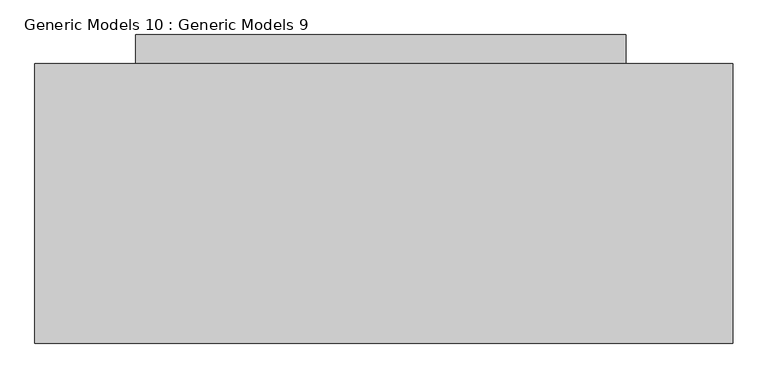
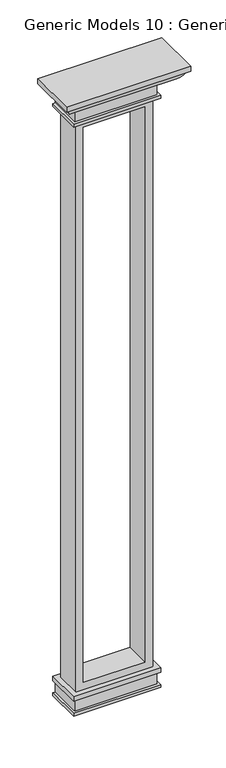
"""IFC4 building model written with IfcOpenShell, lengths in millimetres: proxy geometry, Generic Models 10 : Generic Models 9."""

from ifc_helpers import new_model, si_unit, frame, origin, place, context, project, spatial, polyline, circle_curve, ellipse_curve, outline, extrude, faceted_brep, source, transform, mapped, element, save
from ifc_brep_helpers import plane_surface, cylinder_surface, advanced_brep


def generic_models_10_generic_models_9_50d809b8(model_context):
    return source(origin(), model_context, "Body", "SolidModel", [
        faceted_brep([(-8583.4825076, -5191.2608295, 25.4), (-7719.8825076, -5191.2608295, 25.4), (-7719.8825076, -4835.6608295, 25.4), (-8583.4825076, -4835.6608295, 25.4), (-8583.4825076, -5191.2608295, -177.8), (-8583.4825076, -4835.6608295, -177.8), (-7719.8825076, -4835.6608295, -177.8), (-7719.8825076, -5191.2608295, -177.8), (-8583.4825076, -5191.2608295, -21.3402657), (-7719.8825076, -5191.2608295, -21.3402657), (-7719.8825076, -5191.2608295, -148.3402657), (-8583.4825076, -5191.2608295, -148.3402657), (-7719.8825076, -4835.6608295, -21.3402657), (-7719.8825076, -4835.6608295, -148.3402657), (-7745.2825076, -4835.6608295, -21.3402657), (-7745.2825076, -4835.6608295, -148.3402657), (-8583.4825076, -4835.6608295, -148.3402657), (-8558.0825076, -4835.6608295, -148.3402657), (-8558.0825076, -4835.6608295, -21.3402657), (-8583.4825076, -4835.6608295, -21.3402657), (-8558.0825076, -5165.8608295, -148.3402657), (-8558.0825076, -5165.8608295, -21.3402657), (-7745.2825076, -5165.8608295, -148.3402657), (-7745.2825076, -5165.8608295, -21.3402657)], [[[0, 1, 2, 3]], [[4, 5, 6, 7]], [[1, 0, 8, 9]], [[4, 7, 10, 11]], [[2, 1, 9, 12]], [[7, 6, 13, 10]], [[3, 2, 12, 14, 15, 13, 6, 5, 16, 17, 18, 19]], [[0, 3, 19, 8]], [[5, 4, 11, 16]], [[17, 20, 21, 18]], [[20, 17, 16, 11, 10, 13, 15, 22]], [[18, 21, 23, 14, 12, 9, 8, 19]], [[21, 20, 22, 23]], [[22, 15, 14, 23]]]),
        advanced_brep(
        [(-7531.7890718, -4886.4608295, 6375.4), (-8761.2825076, -4886.4608295, 6375.4), (-8761.2825076, -5379.3542653, 6375.4), (-7531.7890718, -5379.3542653, 6375.4), (-8588.9147157, -4886.4608295, 6197.6), (-8583.4825076, -4886.4608295, 6197.6), (-7709.5890718, -4886.4608295, 6197.6), (-7704.1568638, -4886.4608295, 6197.6), (-7704.1568638, -5206.9864733, 6197.6), (-8588.9147157, -5206.9864733, 6197.6), (-7531.7890718, -4886.4608295, 6324.6), (-7557.1890718, -4886.4608295, 6324.6), (-8735.8825076, -4886.4608295, 6324.6), (-8761.2825076, -4886.4608295, 6324.6), (-8735.8825076, -5353.9542653, 6324.6), (-7557.1890718, -5353.9542653, 6324.6), (-7531.7890718, -5379.3542653, 6324.6), (-8761.2825076, -5379.3542653, 6324.6)],
        [
            (0, 1),
            (1, 2),
            (2, 3),
            (3, 0),
            (4, 5),
            (5, 6),
            (6, 7),
            (7, 8),
            (8, 9),
            (9, 4),
            (0, 10),
            (10, 11),
            (11, 7, circle_curve(frame((-7706.8729678, -4886.4608295, 6349.2806752), z_axis=(0.0, 1.0, 0.0), x_axis=(-1.0, 0.0, 0.0)), 151.7049915)),
            (4, 12, circle_curve(frame((-8586.1986116, -4886.4608295, 6349.2806752), z_axis=(0.0, 1.0, 0.0), x_axis=(1.0, 0.0, 0.0)), 151.7049915)),
            (12, 13),
            (13, 1),
            (12, 14),
            (14, 15),
            (15, 11),
            (10, 16),
            (16, 17),
            (17, 13),
            (9, 14, ellipse_curve(frame((-8586.1986116, -5204.2703693, 6349.2806752), z_axis=(-0.7071067811865468, 0.7071067811865481, 0.0), x_axis=(-0.707106781186548, -0.7071067811865469, 0.0)), 214.5432564, 151.7049915)),
            (17, 2),
            (8, 15, ellipse_curve(frame((-7706.8729678, -5204.2703693, 6349.2806752), z_axis=(-0.7071067811865475, -0.7071067811865475, 0.0), x_axis=(0.7071067811865477, -0.7071067811865474, 0.0)), 214.5432564, 151.7049915)),
            (16, 3),
        ],
        [
            plane_surface(frame((-7465.8825076, -5445.2608295, 6375.4), z_axis=(0.0, 0.0, 1.0), x_axis=(1.0, 0.0, 0.0))),
            plane_surface(frame((-7465.8825076, -5445.2608295, 6197.6), z_axis=(0.0, 0.0, -1.0), x_axis=(-1.0, 0.0, 0.0))),
            plane_surface(frame((-7465.8825076, -4886.4608295, 6375.4), z_axis=(0.0, 1.0, 0.0), x_axis=(0.0, 0.0, -1.0))),
            plane_surface(frame((-8761.2825076, -4886.4608295, 6324.6), z_axis=(0.0, 0.0, -1.0), x_axis=(0.0, -1.0, 0.0))),
            cylinder_surface(frame((-8586.1986116, -4886.4608295, 6349.2806752), z_axis=(0.0, -1.0, 0.0), x_axis=(1.0, 0.0, 0.0)), 151.7049915),
            plane_surface(frame((-8761.2825076, -4886.4608295, 6375.4), z_axis=(-1.0, 0.0, 0.0), x_axis=(0.0, -1.0, 0.0))),
            cylinder_surface(frame((-8827.1890718, -5204.2703693, 6349.2806752), z_axis=(1.0, 0.0, 0.0), x_axis=(0.0, 1.0, 0.0)), 151.7049915),
            plane_surface(frame((-8761.2825076, -5379.3542653, 6375.4), z_axis=(0.0, -1.0, 0.0), x_axis=(1.0, 0.0, 0.0))),
            cylinder_surface(frame((-7706.8729678, -5445.2608295, 6349.2806752), z_axis=(0.0, 1.0, 0.0), x_axis=(-1.0, 0.0, 0.0)), 151.7049915),
            plane_surface(frame((-7531.7890718, -5379.3542653, 6375.4), z_axis=(1.0, 0.0, 0.0), x_axis=(0.0, 1.0, 0.0))),
        ],
        [
            (0, [[1, 2, 3, 4]]),
            (1, [[5, 6, 7, 8, 9, 10]]),
            (2, [[-1, 11, 12, 13, -7, -6, -5, 14, 15, 16]]),
            (3, [[17, 18, 19, -12, 20, 21, 22, -15]]),
            (4, [[-17, -14, -10, 23]]),
            (5, [[-22, 24, -2, -16]]),
            (6, [[-18, -23, -9, 25]]),
            (7, [[-21, 26, -3, -24]]),
            (8, [[-19, -25, -8, -13]]),
            (9, [[-20, -11, -4, -26]]),
        ],
    ),
        faceted_brep([(-8583.4825076, -5191.2608295, 6197.6), (-7719.8825076, -5191.2608295, 6197.6), (-7719.8825076, -4835.6608295, 6197.6), (-8583.4825076, -4835.6608295, 6197.6), (-8583.4825076, -4886.4608295, 6197.6), (-8583.4825076, -5191.2608295, 5994.4), (-8583.4825076, -4835.6608295, 5994.4), (-7719.8825076, -4835.6608295, 5994.4), (-7719.8825076, -5191.2608295, 5994.4), (-8583.4825076, -5191.2608295, 6150.8597343), (-7719.8825076, -5191.2608295, 6150.8597343), (-7719.8825076, -5191.2608295, 6023.8597343), (-8583.4825076, -5191.2608295, 6023.8597343), (-7719.8825076, -4835.6608295, 6150.8597343), (-7719.8825076, -4835.6608295, 6023.8597343), (-7745.2825076, -4835.6608295, 6150.8597343), (-7745.2825076, -4835.6608295, 6023.8597343), (-8583.4825076, -4835.6608295, 6023.8597343), (-8558.0825076, -4835.6608295, 6023.8597343), (-8558.0825076, -4835.6608295, 6150.8597343), (-8583.4825076, -4835.6608295, 6150.8597343), (-8583.4825076, -4886.4608295, 6150.8597343), (-8558.0825076, -5165.8608295, 6023.8597343), (-8558.0825076, -5165.8608295, 6150.8597343), (-7745.2825076, -5165.8608295, 6023.8597343), (-7745.2825076, -5165.8608295, 6150.8597343)], [[[0, 1, 2, 3, 4]], [[5, 6, 7, 8]], [[1, 0, 9, 10]], [[5, 8, 11, 12]], [[2, 1, 10, 13]], [[8, 7, 14, 11]], [[3, 2, 13, 15, 16, 14, 7, 6, 17, 18, 19, 20]], [[6, 5, 12, 17]], [[9, 0, 4, 3, 20, 21]], [[18, 22, 23, 19]], [[22, 18, 17, 12, 11, 14, 16, 24]], [[19, 23, 25, 15, 13, 10, 9, 21, 20]], [[23, 22, 24, 25]], [[24, 16, 15, 25]]]),
        extrude(outline(polyline([(5994.4, -7770.6825076), (5994.4, -8532.6825076), (25.4, -8532.6825076), (25.4, -7770.6825076), (5994.4, -7770.6825076)]), holes=[polyline([(5918.2, -8456.4825076), (5918.2, -7846.8825076), (101.6, -7846.8825076), (101.6, -8456.4825076), (5918.2, -8456.4825076)])]), frame((0.0, -5140.4608295, 0.0), z_axis=(0.0, 1.0, 0.0), x_axis=(0.0, 0.0, 1.0)), (0.0, 0.0, 1.0), 254.0),
    ])


if __name__ == "__main__":
    model = new_model("IFC4")
    model_context = context("Model", 3, world=origin())
    ifc_project = project(units=[si_unit("LENGTHUNIT", "METRE", prefix="MILLI")], contexts=[model_context])
    site = spatial("IfcSite", under=ifc_project)
    building = spatial("IfcBuilding", under=site)
    placement = place(None, origin())
    generic_models_10_generic_models_9_shape = generic_models_10_generic_models_9_50d809b8(model_context)
    element("IfcBuildingElementProxy", 1, Name="Generic Models 10 : Generic Models 9", ObjectType="Generic Models 10 : Generic Models 9", at=placement, inside=building, context=model_context, shape_type="MappedRepresentation", body=[
        mapped(generic_models_10_generic_models_9_shape, transform((0.0, 0.0, 0.0), x_axis=(1.0, 0.0, 0.0), y_axis=(0.0, 1.0, 0.0), z_axis=(0.0, 0.0, 1.0))),
    ])
    save(model, "model.ifc")
